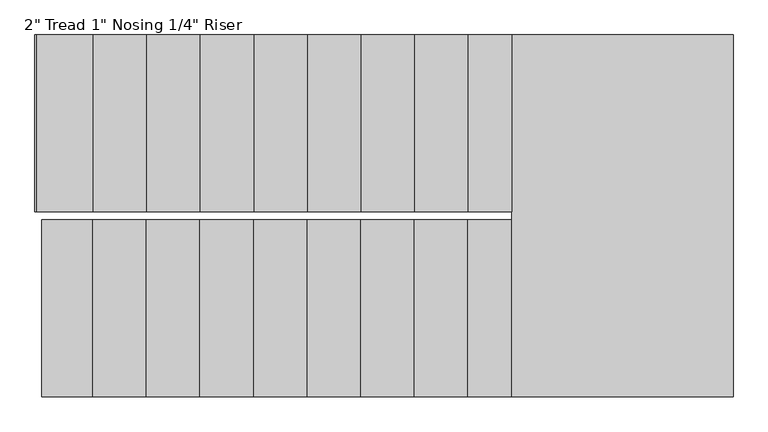
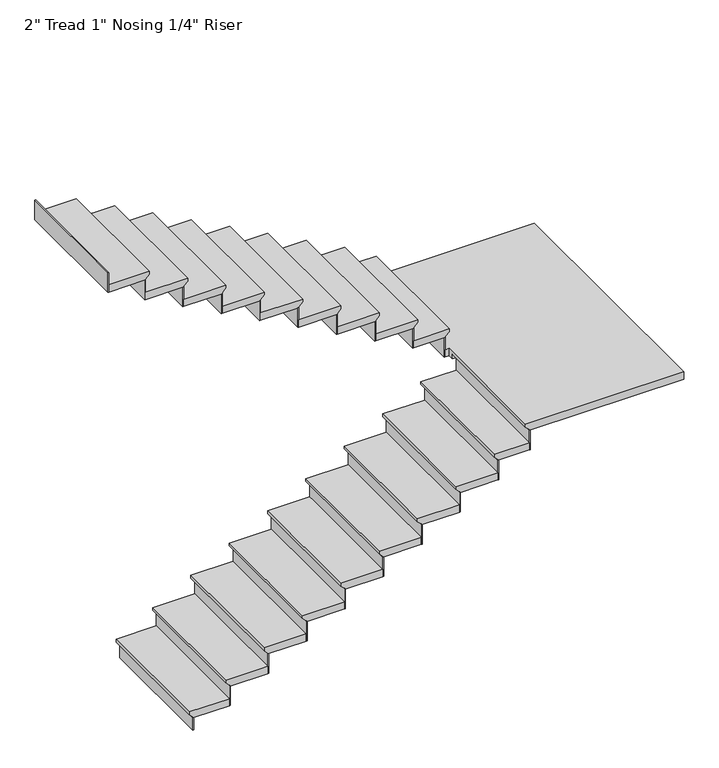
"""IFC4 building model written with IfcOpenShell, lengths in millimetres: stair flight geometry."""

from ifc_helpers import new_model, si_unit, origin, place, context, project, spatial, faceted_brep, source, transform, mapped, element, save


def stair_flight_45fd387a(model_context):
    return source(origin(), model_context, "Body", "Brep", [
        faceted_brep([(-1903.1876145, -1606.0595056, 3166.11), (-1903.1876145, -1606.0595056, 3185.16), (-1903.1876145, -767.8595056, 3185.16), (-1903.1876145, -767.8595056, 3166.11), (-1877.7876145, -1606.0595056, 3140.71), (-1877.7876145, -767.8595056, 3140.71), (-1635.543606, -1606.0595056, 3185.16), (-1635.543606, -767.8595056, 3185.16), (-1877.7876145, -767.8595056, 3134.36), (-1635.543606, -767.8595056, 3134.36), (-1635.543606, -1606.0595056, 3134.36), (-1877.7876145, -1606.0595056, 3134.36)], [[[0, 1, 2, 3]], [[4, 0, 3, 5]], [[2, 1, 6, 7]], [[8, 9, 10, 11]], [[2, 7, 9, 8, 5, 3]], [[8, 11, 4, 5]], [[6, 1, 0, 4, 11, 10]], [[7, 6, 10, 9]]]),
        faceted_brep([(-1877.7876145, -1606.0595056, 3134.36), (-1877.7876145, -1606.0595056, 3048.0), (-1871.4376145, -1606.0595056, 3048.0), (-1871.4376145, -1606.0595056, 3134.36), (-1877.7876145, -767.8595056, 3134.36), (-1871.4376145, -767.8595056, 3134.36), (-1871.4376145, -767.8595056, 3048.0), (-1877.7876145, -767.8595056, 3048.0)], [[[0, 1, 2, 3]], [[4, 5, 6, 7]], [[1, 0, 4, 7]], [[2, 1, 7, 6]], [[3, 2, 6, 5]], [[0, 3, 5, 4]]]),
        faceted_brep([(-1635.543606, -1606.0595056, 3271.52), (-1635.543606, -1606.0595056, 3134.36), (-1629.193606, -1606.0595056, 3134.36), (-1629.193606, -1606.0595056, 3271.52), (-1635.543606, -767.8595056, 3271.52), (-1629.193606, -767.8595056, 3271.52), (-1629.193606, -767.8595056, 3134.36), (-1635.543606, -767.8595056, 3134.36)], [[[0, 1, 2, 3]], [[4, 5, 6, 7]], [[1, 0, 4, 7]], [[2, 1, 7, 6]], [[3, 2, 6, 5]], [[0, 3, 5, 4]]]),
        faceted_brep([(-1660.943606, -767.8595056, 3322.32), (-1660.943606, -1606.0595056, 3322.32), (-1381.543606, -1606.0595056, 3322.32), (-1381.543606, -767.8595056, 3322.32), (-1635.543606, -767.8595056, 3271.52), (-1381.543606, -767.8595056, 3271.52), (-1381.543606, -1606.0595056, 3271.52), (-1635.543606, -1606.0595056, 3271.52), (-1635.543606, -767.8595056, 3277.87), (-1660.943606, -767.8595056, 3303.27), (-1635.543606, -1606.0595056, 3277.87), (-1660.943606, -1606.0595056, 3303.27)], [[[0, 1, 2, 3]], [[4, 5, 6, 7]], [[0, 3, 5, 4, 8, 9]], [[4, 7, 10, 8]], [[2, 1, 11, 10, 7, 6]], [[3, 2, 6, 5]], [[11, 1, 0, 9]], [[10, 11, 9, 8]]]),
        faceted_brep([(-1381.543606, -1606.0595056, 3408.68), (-1381.543606, -1606.0595056, 3271.52), (-1375.193606, -1606.0595056, 3271.52), (-1375.193606, -1606.0595056, 3408.68), (-1381.543606, -767.8595056, 3408.68), (-1375.193606, -767.8595056, 3408.68), (-1375.193606, -767.8595056, 3271.52), (-1381.543606, -767.8595056, 3271.52)], [[[0, 1, 2, 3]], [[4, 5, 6, 7]], [[1, 0, 4, 7]], [[2, 1, 7, 6]], [[3, 2, 6, 5]], [[0, 3, 5, 4]]]),
        faceted_brep([(-1406.943606, -767.8595056, 3459.48), (-1406.943606, -1606.0595056, 3459.48), (-1127.543606, -1606.0595056, 3459.48), (-1127.543606, -767.8595056, 3459.48), (-1381.543606, -767.8595056, 3408.68), (-1127.543606, -767.8595056, 3408.68), (-1127.543606, -1606.0595056, 3408.68), (-1381.543606, -1606.0595056, 3408.68), (-1381.543606, -767.8595056, 3415.03), (-1406.943606, -767.8595056, 3440.43), (-1381.543606, -1606.0595056, 3415.03), (-1406.943606, -1606.0595056, 3440.43)], [[[0, 1, 2, 3]], [[4, 5, 6, 7]], [[0, 3, 5, 4, 8, 9]], [[4, 7, 10, 8]], [[2, 1, 11, 10, 7, 6]], [[3, 2, 6, 5]], [[11, 1, 0, 9]], [[10, 11, 9, 8]]]),
        faceted_brep([(-1127.543606, -1606.0595056, 3545.84), (-1127.543606, -1606.0595056, 3408.68), (-1121.193606, -1606.0595056, 3408.68), (-1121.193606, -1606.0595056, 3545.84), (-1127.543606, -767.8595056, 3545.84), (-1121.193606, -767.8595056, 3545.84), (-1121.193606, -767.8595056, 3408.68), (-1127.543606, -767.8595056, 3408.68)], [[[0, 1, 2, 3]], [[4, 5, 6, 7]], [[1, 0, 4, 7]], [[2, 1, 7, 6]], [[3, 2, 6, 5]], [[0, 3, 5, 4]]]),
        faceted_brep([(-1152.943606, -767.8595056, 3596.64), (-1152.943606, -1606.0595056, 3596.64), (-873.543606, -1606.0595056, 3596.64), (-873.543606, -767.8595056, 3596.64), (-1127.543606, -767.8595056, 3545.84), (-873.543606, -767.8595056, 3545.84), (-873.543606, -1606.0595056, 3545.84), (-1127.543606, -1606.0595056, 3545.84), (-1127.543606, -767.8595056, 3552.19), (-1152.943606, -767.8595056, 3577.59), (-1127.543606, -1606.0595056, 3552.19), (-1152.943606, -1606.0595056, 3577.59)], [[[0, 1, 2, 3]], [[4, 5, 6, 7]], [[0, 3, 5, 4, 8, 9]], [[4, 7, 10, 8]], [[2, 1, 11, 10, 7, 6]], [[3, 2, 6, 5]], [[11, 1, 0, 9]], [[10, 11, 9, 8]]]),
        faceted_brep([(-873.543606, -1606.0595056, 3683.0), (-873.543606, -1606.0595056, 3545.84), (-867.193606, -1606.0595056, 3545.84), (-867.193606, -1606.0595056, 3683.0), (-873.543606, -767.8595056, 3683.0), (-867.193606, -767.8595056, 3683.0), (-867.193606, -767.8595056, 3545.84), (-873.543606, -767.8595056, 3545.84)], [[[0, 1, 2, 3]], [[4, 5, 6, 7]], [[1, 0, 4, 7]], [[2, 1, 7, 6]], [[3, 2, 6, 5]], [[0, 3, 5, 4]]]),
        faceted_brep([(-898.943606, -767.8595056, 3733.8), (-898.943606, -1606.0595056, 3733.8), (-619.543606, -1606.0595056, 3733.8), (-619.543606, -767.8595056, 3733.8), (-873.543606, -767.8595056, 3683.0), (-619.543606, -767.8595056, 3683.0), (-619.543606, -1606.0595056, 3683.0), (-873.543606, -1606.0595056, 3683.0), (-873.543606, -767.8595056, 3689.35), (-898.943606, -767.8595056, 3714.75), (-873.543606, -1606.0595056, 3689.35), (-898.943606, -1606.0595056, 3714.75)], [[[0, 1, 2, 3]], [[4, 5, 6, 7]], [[0, 3, 5, 4, 8, 9]], [[4, 7, 10, 8]], [[2, 1, 11, 10, 7, 6]], [[3, 2, 6, 5]], [[11, 1, 0, 9]], [[10, 11, 9, 8]]]),
        faceted_brep([(-619.543606, -1606.0595056, 3820.16), (-619.543606, -1606.0595056, 3683.0), (-613.193606, -1606.0595056, 3683.0), (-613.193606, -1606.0595056, 3820.16), (-619.543606, -767.8595056, 3820.16), (-613.193606, -767.8595056, 3820.16), (-613.193606, -767.8595056, 3683.0), (-619.543606, -767.8595056, 3683.0)], [[[0, 1, 2, 3]], [[4, 5, 6, 7]], [[1, 0, 4, 7]], [[2, 1, 7, 6]], [[3, 2, 6, 5]], [[0, 3, 5, 4]]]),
        faceted_brep([(-644.943606, -767.8595056, 3870.96), (-644.943606, -1606.0595056, 3870.96), (-365.543606, -1606.0595056, 3870.96), (-365.543606, -767.8595056, 3870.96), (-619.543606, -767.8595056, 3820.16), (-365.543606, -767.8595056, 3820.16), (-365.543606, -1606.0595056, 3820.16), (-619.543606, -1606.0595056, 3820.16), (-619.543606, -767.8595056, 3826.51), (-644.943606, -767.8595056, 3851.91), (-619.543606, -1606.0595056, 3826.51), (-644.943606, -1606.0595056, 3851.91)], [[[0, 1, 2, 3]], [[4, 5, 6, 7]], [[0, 3, 5, 4, 8, 9]], [[4, 7, 10, 8]], [[2, 1, 11, 10, 7, 6]], [[3, 2, 6, 5]], [[11, 1, 0, 9]], [[10, 11, 9, 8]]]),
        faceted_brep([(-365.543606, -1606.0595056, 3957.32), (-365.543606, -1606.0595056, 3820.16), (-359.193606, -1606.0595056, 3820.16), (-359.193606, -1606.0595056, 3957.32), (-365.543606, -767.8595056, 3957.32), (-359.193606, -767.8595056, 3957.32), (-359.193606, -767.8595056, 3820.16), (-365.543606, -767.8595056, 3820.16)], [[[0, 1, 2, 3]], [[4, 5, 6, 7]], [[1, 0, 4, 7]], [[2, 1, 7, 6]], [[3, 2, 6, 5]], [[0, 3, 5, 4]]]),
        faceted_brep([(-390.943606, -767.8595056, 4008.12), (-390.943606, -1606.0595056, 4008.12), (-111.543606, -1606.0595056, 4008.12), (-111.543606, -767.8595056, 4008.12), (-365.543606, -767.8595056, 3957.32), (-111.543606, -767.8595056, 3957.32), (-111.543606, -1606.0595056, 3957.32), (-365.543606, -1606.0595056, 3957.32), (-365.543606, -767.8595056, 3963.67), (-390.943606, -767.8595056, 3989.07), (-365.543606, -1606.0595056, 3963.67), (-390.943606, -1606.0595056, 3989.07)], [[[0, 1, 2, 3]], [[4, 5, 6, 7]], [[0, 3, 5, 4, 8, 9]], [[4, 7, 10, 8]], [[2, 1, 11, 10, 7, 6]], [[3, 2, 6, 5]], [[11, 1, 0, 9]], [[10, 11, 9, 8]]]),
        faceted_brep([(-111.543606, -1606.0595056, 4094.48), (-111.543606, -1606.0595056, 3957.32), (-105.193606, -1606.0595056, 3957.32), (-105.193606, -1606.0595056, 4094.48), (-111.543606, -767.8595056, 4094.48), (-105.193606, -767.8595056, 4094.48), (-105.193606, -767.8595056, 3957.32), (-111.543606, -767.8595056, 3957.32)], [[[0, 1, 2, 3]], [[4, 5, 6, 7]], [[1, 0, 4, 7]], [[2, 1, 7, 6]], [[3, 2, 6, 5]], [[0, 3, 5, 4]]]),
        faceted_brep([(-136.943606, -767.8595056, 4145.28), (-136.943606, -1606.0595056, 4145.28), (142.456394, -1606.0595056, 4145.28), (142.456394, -767.8595056, 4145.28), (-111.543606, -767.8595056, 4094.48), (142.456394, -767.8595056, 4094.48), (142.456394, -1606.0595056, 4094.48), (-111.543606, -1606.0595056, 4094.48), (-111.543606, -767.8595056, 4100.83), (-136.943606, -767.8595056, 4126.23), (-111.543606, -1606.0595056, 4100.83), (-136.943606, -1606.0595056, 4126.23)], [[[0, 1, 2, 3]], [[4, 5, 6, 7]], [[0, 3, 5, 4, 8, 9]], [[4, 7, 10, 8]], [[2, 1, 11, 10, 7, 6]], [[3, 2, 6, 5]], [[11, 1, 0, 9]], [[10, 11, 9, 8]]]),
        faceted_brep([(142.456394, -1606.0595056, 4231.64), (142.456394, -1606.0595056, 4094.48), (148.806394, -1606.0595056, 4094.48), (148.806394, -1606.0595056, 4231.64), (142.456394, -767.8595056, 4231.64), (148.806394, -767.8595056, 4231.64), (148.806394, -767.8595056, 4094.48), (142.456394, -767.8595056, 4094.48)], [[[0, 1, 2, 3]], [[4, 5, 6, 7]], [[1, 0, 4, 7]], [[2, 1, 7, 6]], [[3, 2, 6, 5]], [[0, 3, 5, 4]]]),
        faceted_brep([(117.056394, -767.8595056, 4282.44), (117.056394, -1606.0595056, 4282.44), (350.8830625, -1606.0595056, 4282.44), (350.8830625, -767.8595056, 4282.44), (142.456394, -767.8595056, 4231.64), (350.8830625, -767.8595056, 4231.64), (350.8830625, -1606.0595056, 4231.64), (142.456394, -1606.0595056, 4231.64), (142.456394, -767.8595056, 4237.99), (117.056394, -767.8595056, 4263.39), (142.456394, -1606.0595056, 4237.99), (117.056394, -1606.0595056, 4263.39)], [[[0, 1, 2, 3]], [[4, 5, 6, 7]], [[0, 3, 5, 4, 8, 9]], [[4, 7, 10, 8]], [[2, 1, 11, 10, 7, 6]], [[3, 2, 6, 5]], [[11, 1, 0, 9]], [[10, 11, 9, 8]]]),
        faceted_brep([(350.8830625, -1606.0595056, 4368.8), (350.8830625, -1606.0595056, 4231.64), (357.2330625, -1606.0595056, 4231.64), (357.2330625, -1606.0595056, 4368.8), (350.8830625, -767.8595056, 4368.8), (357.2330625, -767.8595056, 4368.8), (357.2330625, -767.8595056, 4231.64), (350.8830625, -767.8595056, 4231.64)], [[[0, 1, 2, 3]], [[4, 5, 6, 7]], [[1, 0, 4, 7]], [[2, 1, 7, 6]], [[3, 2, 6, 5]], [[0, 3, 5, 4]]]),
        faceted_brep([(300.0830625, -729.7595056, 4419.6), (325.4830625, -729.7595056, 4419.6), (325.4830625, -1606.0595056, 4419.6), (1373.4123855, -1606.0595056, 4419.6), (1373.4123855, 108.4404944, 4419.6), (300.0830625, 108.4404944, 4419.6), (325.4830625, -729.7595056, 4368.8), (300.0830625, -729.7595056, 4368.8), (300.0830625, 108.4404944, 4368.8), (1373.4123855, 108.4404944, 4368.8), (1373.4123855, -1606.0595056, 4368.8), (350.8830625, -1606.0595056, 4368.8), (350.8830625, -767.8595056, 4368.8), (325.4830625, -767.8595056, 4368.8), (325.4830625, -767.8595056, 4400.55), (325.4830625, -1606.0595056, 4400.55), (350.8830625, -767.8595056, 4375.15), (350.8830625, -1606.0595056, 4375.15)], [[[0, 1, 2, 3, 4, 5]], [[6, 7, 8, 9, 10, 11, 12, 13]], [[1, 0, 7, 6]], [[2, 1, 6, 13, 14, 15]], [[13, 12, 16, 14]], [[12, 11, 17, 16]], [[3, 2, 15, 17, 11, 10]], [[4, 3, 10, 9]], [[5, 4, 9, 8]], [[0, 5, 8, 7]], [[17, 15, 14, 16]]]),
        faceted_brep([(300.0830625, 108.4404944, 4505.96), (300.0830625, 108.4404944, 4368.8), (293.7330625, 108.4404944, 4368.8), (293.7330625, 108.4404944, 4505.96), (300.0830625, -729.7595056, 4505.96), (293.7330625, -729.7595056, 4505.96), (293.7330625, -729.7595056, 4368.8), (300.0830625, -729.7595056, 4368.8)], [[[0, 1, 2, 3]], [[4, 5, 6, 7]], [[1, 0, 4, 7]], [[2, 1, 7, 6]], [[3, 2, 6, 5]], [[0, 3, 5, 4]]]),
        faceted_brep([(325.4830625, -729.7595056, 4556.76), (325.4830625, 108.4404944, 4556.76), (91.656394, 108.4404944, 4556.76), (91.656394, -729.7595056, 4556.76), (300.0830625, -729.7595056, 4505.96), (91.656394, -729.7595056, 4505.96), (91.656394, 108.4404944, 4505.96), (300.0830625, 108.4404944, 4505.96), (300.0830625, -729.7595056, 4512.31), (325.4830625, -729.7595056, 4537.71), (300.0830625, 108.4404944, 4512.31), (325.4830625, 108.4404944, 4537.71)], [[[0, 1, 2, 3]], [[4, 5, 6, 7]], [[0, 3, 5, 4, 8, 9]], [[4, 7, 10, 8]], [[2, 1, 11, 10, 7, 6]], [[3, 2, 6, 5]], [[11, 1, 0, 9]], [[10, 11, 9, 8]]]),
        faceted_brep([(91.656394, 108.4404944, 4643.12), (91.656394, 108.4404944, 4505.96), (85.306394, 108.4404944, 4505.96), (85.306394, 108.4404944, 4643.12), (91.656394, -729.7595056, 4643.12), (85.306394, -729.7595056, 4643.12), (85.306394, -729.7595056, 4505.96), (91.656394, -729.7595056, 4505.96)], [[[0, 1, 2, 3]], [[4, 5, 6, 7]], [[1, 0, 4, 7]], [[2, 1, 7, 6]], [[3, 2, 6, 5]], [[0, 3, 5, 4]]]),
        faceted_brep([(117.056394, -729.7595056, 4693.92), (117.056394, 108.4404944, 4693.92), (-162.343606, 108.4404944, 4693.92), (-162.343606, -729.7595056, 4693.92), (91.656394, -729.7595056, 4643.12), (-162.343606, -729.7595056, 4643.12), (-162.343606, 108.4404944, 4643.12), (91.656394, 108.4404944, 4643.12), (91.656394, -729.7595056, 4649.47), (117.056394, -729.7595056, 4674.87), (91.656394, 108.4404944, 4649.47), (117.056394, 108.4404944, 4674.87)], [[[0, 1, 2, 3]], [[4, 5, 6, 7]], [[0, 3, 5, 4, 8, 9]], [[4, 7, 10, 8]], [[2, 1, 11, 10, 7, 6]], [[3, 2, 6, 5]], [[11, 1, 0, 9]], [[10, 11, 9, 8]]]),
        faceted_brep([(-162.343606, 108.4404944, 4780.28), (-162.343606, 108.4404944, 4643.12), (-168.693606, 108.4404944, 4643.12), (-168.693606, 108.4404944, 4780.28), (-162.343606, -729.7595056, 4780.28), (-168.693606, -729.7595056, 4780.28), (-168.693606, -729.7595056, 4643.12), (-162.343606, -729.7595056, 4643.12)], [[[0, 1, 2, 3]], [[4, 5, 6, 7]], [[1, 0, 4, 7]], [[2, 1, 7, 6]], [[3, 2, 6, 5]], [[0, 3, 5, 4]]]),
        faceted_brep([(-136.943606, -729.7595056, 4831.08), (-136.943606, 108.4404944, 4831.08), (-416.343606, 108.4404944, 4831.08), (-416.343606, -729.7595056, 4831.08), (-162.343606, -729.7595056, 4780.28), (-416.343606, -729.7595056, 4780.28), (-416.343606, 108.4404944, 4780.28), (-162.343606, 108.4404944, 4780.28), (-162.343606, -729.7595056, 4786.63), (-136.943606, -729.7595056, 4812.03), (-162.343606, 108.4404944, 4786.63), (-136.943606, 108.4404944, 4812.03)], [[[0, 1, 2, 3]], [[4, 5, 6, 7]], [[0, 3, 5, 4, 8, 9]], [[4, 7, 10, 8]], [[2, 1, 11, 10, 7, 6]], [[3, 2, 6, 5]], [[11, 1, 0, 9]], [[10, 11, 9, 8]]]),
        faceted_brep([(-416.343606, 108.4404944, 4917.44), (-416.343606, 108.4404944, 4780.28), (-422.693606, 108.4404944, 4780.28), (-422.693606, 108.4404944, 4917.44), (-416.343606, -729.7595056, 4917.44), (-422.693606, -729.7595056, 4917.44), (-422.693606, -729.7595056, 4780.28), (-416.343606, -729.7595056, 4780.28)], [[[0, 1, 2, 3]], [[4, 5, 6, 7]], [[1, 0, 4, 7]], [[2, 1, 7, 6]], [[3, 2, 6, 5]], [[0, 3, 5, 4]]]),
        faceted_brep([(-390.943606, -729.7595056, 4968.24), (-390.943606, 108.4404944, 4968.24), (-670.343606, 108.4404944, 4968.24), (-670.343606, -729.7595056, 4968.24), (-416.343606, -729.7595056, 4917.44), (-670.343606, -729.7595056, 4917.44), (-670.343606, 108.4404944, 4917.44), (-416.343606, 108.4404944, 4917.44), (-416.343606, -729.7595056, 4923.79), (-390.943606, -729.7595056, 4949.19), (-416.343606, 108.4404944, 4923.79), (-390.943606, 108.4404944, 4949.19)], [[[0, 1, 2, 3]], [[4, 5, 6, 7]], [[0, 3, 5, 4, 8, 9]], [[4, 7, 10, 8]], [[2, 1, 11, 10, 7, 6]], [[3, 2, 6, 5]], [[11, 1, 0, 9]], [[10, 11, 9, 8]]]),
        faceted_brep([(-670.343606, 108.4404944, 5054.6), (-670.343606, 108.4404944, 4917.44), (-676.693606, 108.4404944, 4917.44), (-676.693606, 108.4404944, 5054.6), (-670.343606, -729.7595056, 5054.6), (-676.693606, -729.7595056, 5054.6), (-676.693606, -729.7595056, 4917.44), (-670.343606, -729.7595056, 4917.44)], [[[0, 1, 2, 3]], [[4, 5, 6, 7]], [[1, 0, 4, 7]], [[2, 1, 7, 6]], [[3, 2, 6, 5]], [[0, 3, 5, 4]]]),
        faceted_brep([(-644.943606, -729.7595056, 5105.4), (-644.943606, 108.4404944, 5105.4), (-924.343606, 108.4404944, 5105.4), (-924.343606, -729.7595056, 5105.4), (-670.343606, -729.7595056, 5054.6), (-924.343606, -729.7595056, 5054.6), (-924.343606, 108.4404944, 5054.6), (-670.343606, 108.4404944, 5054.6), (-670.343606, -729.7595056, 5060.95), (-644.943606, -729.7595056, 5086.35), (-670.343606, 108.4404944, 5060.95), (-644.943606, 108.4404944, 5086.35)], [[[0, 1, 2, 3]], [[4, 5, 6, 7]], [[0, 3, 5, 4, 8, 9]], [[4, 7, 10, 8]], [[2, 1, 11, 10, 7, 6]], [[3, 2, 6, 5]], [[11, 1, 0, 9]], [[10, 11, 9, 8]]]),
        faceted_brep([(-924.343606, 108.4404944, 5191.76), (-924.343606, 108.4404944, 5054.6), (-930.693606, 108.4404944, 5054.6), (-930.693606, 108.4404944, 5191.76), (-924.343606, -729.7595056, 5191.76), (-930.693606, -729.7595056, 5191.76), (-930.693606, -729.7595056, 5054.6), (-924.343606, -729.7595056, 5054.6)], [[[0, 1, 2, 3]], [[4, 5, 6, 7]], [[1, 0, 4, 7]], [[2, 1, 7, 6]], [[3, 2, 6, 5]], [[0, 3, 5, 4]]]),
        faceted_brep([(-898.943606, -729.7595056, 5242.56), (-898.943606, 108.4404944, 5242.56), (-1178.343606, 108.4404944, 5242.56), (-1178.343606, -729.7595056, 5242.56), (-924.343606, -729.7595056, 5191.76), (-1178.343606, -729.7595056, 5191.76), (-1178.343606, 108.4404944, 5191.76), (-924.343606, 108.4404944, 5191.76), (-924.343606, -729.7595056, 5198.11), (-898.943606, -729.7595056, 5223.51), (-924.343606, 108.4404944, 5198.11), (-898.943606, 108.4404944, 5223.51)], [[[0, 1, 2, 3]], [[4, 5, 6, 7]], [[0, 3, 5, 4, 8, 9]], [[4, 7, 10, 8]], [[2, 1, 11, 10, 7, 6]], [[3, 2, 6, 5]], [[11, 1, 0, 9]], [[10, 11, 9, 8]]]),
        faceted_brep([(-1178.343606, 108.4404944, 5328.92), (-1178.343606, 108.4404944, 5191.76), (-1184.693606, 108.4404944, 5191.76), (-1184.693606, 108.4404944, 5328.92), (-1178.343606, -729.7595056, 5328.92), (-1184.693606, -729.7595056, 5328.92), (-1184.693606, -729.7595056, 5191.76), (-1178.343606, -729.7595056, 5191.76)], [[[0, 1, 2, 3]], [[4, 5, 6, 7]], [[1, 0, 4, 7]], [[2, 1, 7, 6]], [[3, 2, 6, 5]], [[0, 3, 5, 4]]]),
        faceted_brep([(-1152.943606, -729.7595056, 5379.72), (-1152.943606, 108.4404944, 5379.72), (-1432.343606, 108.4404944, 5379.72), (-1432.343606, -729.7595056, 5379.72), (-1178.343606, -729.7595056, 5328.92), (-1432.343606, -729.7595056, 5328.92), (-1432.343606, 108.4404944, 5328.92), (-1178.343606, 108.4404944, 5328.92), (-1178.343606, -729.7595056, 5335.27), (-1152.943606, -729.7595056, 5360.67), (-1178.343606, 108.4404944, 5335.27), (-1152.943606, 108.4404944, 5360.67)], [[[0, 1, 2, 3]], [[4, 5, 6, 7]], [[0, 3, 5, 4, 8, 9]], [[4, 7, 10, 8]], [[2, 1, 11, 10, 7, 6]], [[3, 2, 6, 5]], [[11, 1, 0, 9]], [[10, 11, 9, 8]]]),
        faceted_brep([(-1432.343606, 108.4404944, 5466.08), (-1432.343606, 108.4404944, 5328.92), (-1438.693606, 108.4404944, 5328.92), (-1438.693606, 108.4404944, 5466.08), (-1432.343606, -729.7595056, 5466.08), (-1438.693606, -729.7595056, 5466.08), (-1438.693606, -729.7595056, 5328.92), (-1432.343606, -729.7595056, 5328.92)], [[[0, 1, 2, 3]], [[4, 5, 6, 7]], [[1, 0, 4, 7]], [[2, 1, 7, 6]], [[3, 2, 6, 5]], [[0, 3, 5, 4]]]),
        faceted_brep([(-1406.943606, -729.7595056, 5516.88), (-1406.943606, 108.4404944, 5516.88), (-1686.343606, 108.4404944, 5516.88), (-1686.343606, -729.7595056, 5516.88), (-1432.343606, -729.7595056, 5466.08), (-1686.343606, -729.7595056, 5466.08), (-1686.343606, 108.4404944, 5466.08), (-1432.343606, 108.4404944, 5466.08), (-1432.343606, -729.7595056, 5472.43), (-1406.943606, -729.7595056, 5497.83), (-1432.343606, 108.4404944, 5472.43), (-1406.943606, 108.4404944, 5497.83)], [[[0, 1, 2, 3]], [[4, 5, 6, 7]], [[0, 3, 5, 4, 8, 9]], [[4, 7, 10, 8]], [[2, 1, 11, 10, 7, 6]], [[3, 2, 6, 5]], [[11, 1, 0, 9]], [[10, 11, 9, 8]]]),
        faceted_brep([(-1686.343606, 108.4404944, 5603.24), (-1686.343606, 108.4404944, 5466.08), (-1692.693606, 108.4404944, 5466.08), (-1692.693606, 108.4404944, 5603.24), (-1686.343606, -729.7595056, 5603.24), (-1692.693606, -729.7595056, 5603.24), (-1692.693606, -729.7595056, 5466.08), (-1686.343606, -729.7595056, 5466.08)], [[[0, 1, 2, 3]], [[4, 5, 6, 7]], [[1, 0, 4, 7]], [[2, 1, 7, 6]], [[3, 2, 6, 5]], [[0, 3, 5, 4]]]),
        faceted_brep([(-1928.5876145, 108.4404944, 5740.4), (-1928.5876145, 108.4404944, 5603.24), (-1934.9376145, 108.4404944, 5603.24), (-1934.9376145, 108.4404944, 5740.4), (-1928.5876145, -729.7595056, 5740.4), (-1934.9376145, -729.7595056, 5740.4), (-1934.9376145, -729.7595056, 5603.24), (-1928.5876145, -729.7595056, 5603.24)], [[[0, 1, 2, 3]], [[4, 5, 6, 7]], [[1, 0, 4, 7]], [[2, 1, 7, 6]], [[3, 2, 6, 5]], [[0, 3, 5, 4]]]),
        faceted_brep([(-1660.943606, -729.7595056, 5654.04), (-1660.943606, 108.4404944, 5654.04), (-1928.5876145, 108.4404944, 5654.04), (-1928.5876145, -729.7595056, 5654.04), (-1686.343606, -729.7595056, 5603.24), (-1928.5876145, -729.7595056, 5603.24), (-1928.5876145, 108.4404944, 5603.24), (-1686.343606, 108.4404944, 5603.24), (-1686.343606, -729.7595056, 5609.59), (-1660.943606, -729.7595056, 5634.99), (-1686.343606, 108.4404944, 5609.59), (-1660.943606, 108.4404944, 5634.99)], [[[0, 1, 2, 3]], [[4, 5, 6, 7]], [[0, 3, 5, 4, 8, 9]], [[4, 7, 10, 8]], [[2, 1, 11, 10, 7, 6]], [[3, 2, 6, 5]], [[11, 1, 0, 9]], [[10, 11, 9, 8]]]),
    ])


if __name__ == "__main__":
    model = new_model("IFC4")
    model_context = context("Model", 3, world=origin())
    ifc_project = project(units=[si_unit("LENGTHUNIT", "METRE", prefix="MILLI")], contexts=[model_context])
    site = spatial("IfcSite", under=ifc_project)
    building = spatial("IfcBuilding", under=site)
    placement = place(None, origin())
    stair_flight_shape = stair_flight_45fd387a(model_context)
    element("IfcStairFlight", 1, ObjectType="2\" Tread 1\" Nosing 1/4\" Riser", at=placement, inside=building, context=model_context, shape_type="MappedRepresentation", body=[
        mapped(stair_flight_shape, transform((0.0, 0.0, 0.0), x_axis=(1.0, 0.0, 0.0), y_axis=(0.0, 1.0, 0.0), z_axis=(0.0, 0.0, 1.0))),
    ])
    save(model, "model.ifc")
